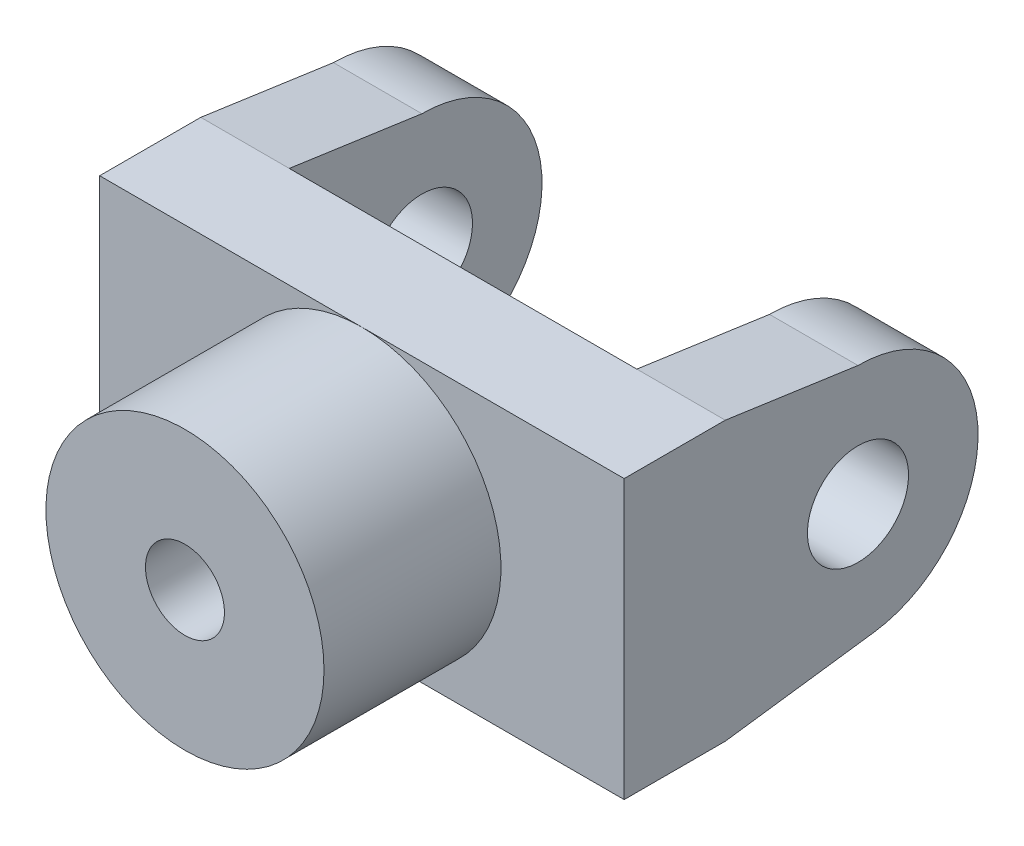
from build123d import *

# Parameters (mm, degrees)
BASE_BLOCK_SKETCH_W         = 166
BASE_BLOCK_SKETCH_H         = 88
BASE_BLOCK_166X88X32_DEPTH  = 32
BORED_BOSS_SKETCH_R         = 44
BORED_BOSS_SKETCH_R_2       = 12.5
BORED_BOSS_88_BORE_25_DEPTH = 56
LUG_SKETCH_R                = 16
PIERCED_LUG_DEPTH           = 28


with BuildPart() as part:
    # Base Block Sketch → Base Block 166x88x32 (new body)
    with BuildSketch(Plane.XY):
        Rectangle(BASE_BLOCK_SKETCH_W, BASE_BLOCK_SKETCH_H)
    extrude(amount=BASE_BLOCK_166X88X32_DEPTH)

    # Bored Boss Sketch → Bored Boss Ø88 Bore Ø25 (add)
    with BuildSketch(Plane.XY.offset(32)):
        with Locations(Location((0, 0, 0), (0, 0, 270))):
            Circle(BORED_BOSS_SKETCH_R)
        Circle(BORED_BOSS_SKETCH_R_2, mode=Mode.SUBTRACT)
    extrude(amount=BORED_BOSS_88_BORE_25_DEPTH)

    # Lug Sketch → Pierced Lug (add)
    with BuildSketch(Plane(origin=(83, 0, 0), x_dir=(0, 0, -1), z_dir=(1, 0, 0))):
        with BuildLine():
            Line((0, 44), (0, -44))
            Line((0, -44), (47.072324291, -37.659945915))
            ThreePointArc((47.072324291, -37.659945915), (79.914891169, 2.541855154), (42, 38))
            Line((42, 38), (0, 44))
        make_face()
        with Locations((42, 0)):
            Circle(LUG_SKETCH_R, mode=Mode.SUBTRACT)
    pierced_lug = extrude(amount=-PIERCED_LUG_DEPTH)

    # Lug Mirror: Pierced Lug across plane
    add(pierced_lug.mirror(Plane(origin=(0, 0, 0), x_dir=(0, 0, 1), z_dir=(1, 0, 0))))


solid = part.part
